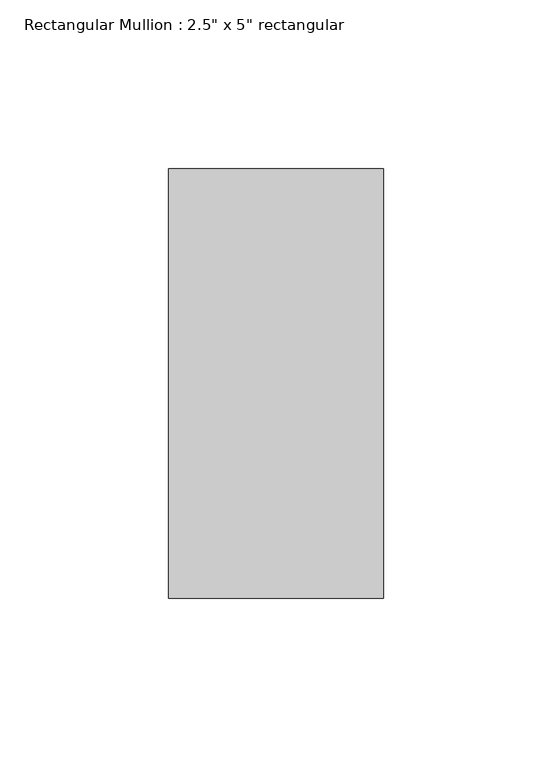
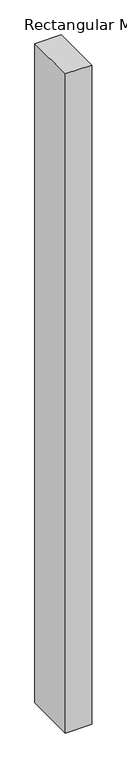
"""IFC4 building model written with IfcOpenShell, lengths in millimetres: member geometry."""

from ifc_helpers import new_model, si_unit, frame, origin, place, context, project, spatial, polyline, outline, extrude, source, transform, mapped, element, save


def member_6b0a351e(model_context):
    return source(origin(), model_context, "Body", "SweptSolid", [
        extrude(outline(polyline([(31.75, 63.5), (31.75, -63.5), (-31.75, -63.5), (-31.75, 63.5), (31.75, 63.5)])), frame((0.0, 0.0, -1675.2875727), z_axis=(0.0, 0.0, 1.0), x_axis=(1.0, 0.0, 0.0)), (0.0, 0.0, 1.0), 1675.2875727),
    ])


if __name__ == "__main__":
    model = new_model("IFC4")
    model_context = context("Model", 3, world=origin())
    ifc_project = project(units=[si_unit("LENGTHUNIT", "METRE", prefix="MILLI")], contexts=[model_context])
    site = spatial("IfcSite", under=ifc_project)
    building = spatial("IfcBuilding", under=site)
    placement = place(None, origin())
    member_shape = member_6b0a351e(model_context)
    element("IfcMember", 1, ObjectType="Rectangular Mullion : 2.5\" x 5\" rectangular", at=placement, inside=building, context=model_context, shape_type="MappedRepresentation", body=[
        mapped(member_shape, transform((0.0, 0.0, 0.0), x_axis=(1.0, 0.0, 0.0), y_axis=(0.0, 1.0, 0.0), z_axis=(0.0, 0.0, 1.0))),
    ])
    save(model, "model.ifc")

# Revit data of these elements
# Type "Rectangular Mullion : 2.5\" x 5\" rectangular"
#   built-in parameter 1007304 = 0.416667 (stored number, unit not read)
#   built-in parameter 1007301 = 0.104167 (stored number, unit not read)
#   built-in parameter 1007300 = 0.104167 (stored number, unit not read)
# Element 1 (IfcMember, "Rectangular Mullion : 2.5\" x 5\" rectangular")
#   Materials on its faces: "Aluminum"
# Materials
#   "Aluminum": class "Metal", colour RGB 247 247 247, transparency 0, Description = "Aluminum 6061", Cost = 0
